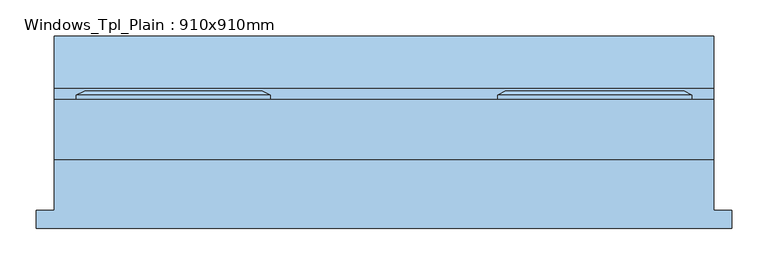
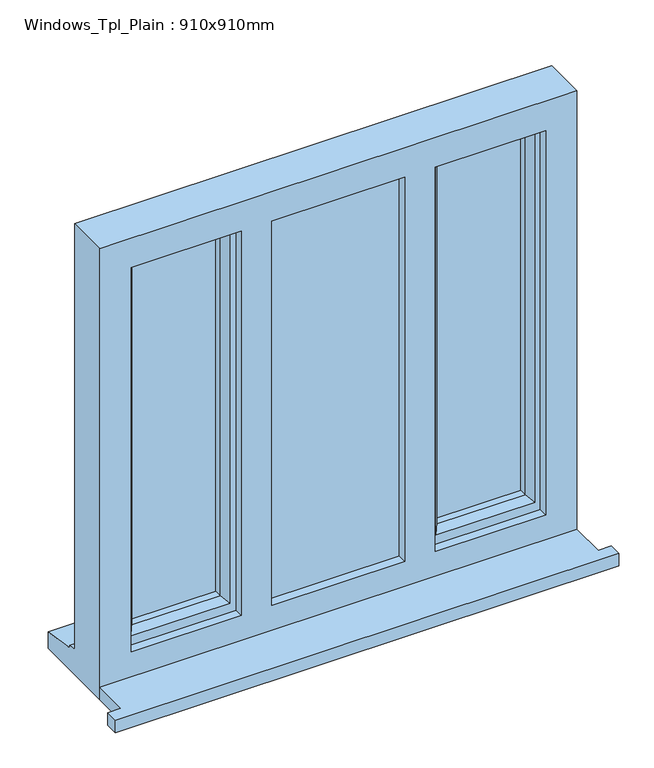
"""IFC4 building model written with IfcOpenShell, lengths in millimetres: window geometry, Windows_Tpl_Plain : 910x910mm."""

from ifc_helpers import new_model, si_unit, frame, origin, place, context, project, spatial, polyline, outline, extrude, faceted_brep, source, transform, mapped, element, save


def windows_tpl_plain_910x910mm_84e79c20(model_context):
    return source(origin(), model_context, "Body", "SolidModel", [
        extrude(outline(polyline([(-906.6666667, -118.1434322), (-906.6666667, -93.1434322), (-881.6666667, -93.1434322), (-881.6666667, -22.9434322), (28.3333333, -22.9434322), (28.3333333, -93.1434322), (53.3333333, -93.1434322), (53.3333333, -118.1434322), (-906.6666667, -118.1434322)])), frame((0.0, 0.0, 1200.0), z_axis=(0.0, 0.0, 1.0), x_axis=(1.0, 0.0, 0.0)), (0.0, 0.0, 1.0), 25.0),
        faceted_brep([(-270.0, 60.0565678, 2080.0), (-270.0, 65.8300705, 2080.0), (-270.0, 65.8300705, 1253.0), (-270.0, 60.0565678, 1253.0), (-260.0, -4.9434322, 2070.0), (-260.0, 60.0565678, 2070.0), (-260.0, 60.0565678, 1263.0), (-260.0, -4.9434322, 1263.0), (-220.0, 9.5494677, 2030.0), (-230.1480377, -4.9434322, 2040.1480377), (-230.1480377, -4.9434322, 1292.8519623), (-220.0, 9.5494677, 1303.0), (-220.0, 24.0565678, 2030.0), (-220.0, 24.0565678, 1303.0), (-230.0, 48.0565678, 2040.0), (-230.0, 24.0565678, 2040.0), (-230.0, 24.0565678, 1293.0), (-230.0, 48.0565678, 1293.0), (-220.0, 65.8300705, 2030.0), (-220.0, 48.0565678, 2030.0), (-220.0, 48.0565678, 1303.0), (-220.0, 65.8300705, 1303.0), (-237.4457548, 71.6035732, 2047.4457548), (-237.4457548, 71.6035732, 1285.5542452), (-259.2153903, 71.6035732, 2069.2153903), (-259.2153903, 71.6035732, 1263.7846097), (-1.6666667, 65.8300705, 1253.0), (-1.6666667, 60.0565678, 1253.0), (-11.6666667, 60.0565678, 1263.0), (-11.6666667, -4.9434322, 1263.0), (-41.5186289, -4.9434322, 1292.8519623), (-51.6666667, 9.5494677, 1303.0), (-51.6666667, 24.0565678, 1303.0), (-41.6666667, 24.0565678, 1293.0), (-41.6666667, 48.0565678, 1293.0), (-51.6666667, 48.0565678, 1303.0), (-51.6666667, 65.8300705, 1303.0), (-34.2209119, 71.6035732, 1285.5542452), (-12.4512764, 71.6035732, 1263.7846097), (-1.6666667, 65.8300705, 2080.0), (-1.6666667, 60.0565678, 2080.0), (-11.6666667, 60.0565678, 2070.0), (-11.6666667, -4.9434322, 2070.0), (-41.5186289, -4.9434322, 2040.1480377), (-51.6666667, 9.5494677, 2030.0), (-51.6666667, 24.0565678, 2030.0), (-41.6666667, 24.0565678, 2040.0), (-41.6666667, 48.0565678, 2040.0), (-51.6666667, 48.0565678, 2030.0), (-51.6666667, 65.8300705, 2030.0), (-34.2209119, 71.6035732, 2047.4457548), (-12.4512764, 71.6035732, 2069.2153903)], [[[0, 1, 2, 3]], [[4, 5, 6, 7]], [[8, 9, 10, 11]], [[12, 8, 11, 13]], [[14, 15, 16, 17]], [[18, 19, 20, 21]], [[22, 18, 21, 23]], [[1, 24, 25, 2]], [[3, 2, 26, 27]], [[7, 6, 28, 29]], [[11, 10, 30, 31]], [[13, 11, 31, 32]], [[17, 16, 33, 34]], [[21, 20, 35, 36]], [[23, 21, 36, 37]], [[2, 25, 38, 26]], [[27, 26, 39, 40]], [[29, 28, 41, 42]], [[31, 30, 43, 44]], [[32, 31, 44, 45]], [[34, 33, 46, 47]], [[36, 35, 48, 49]], [[37, 36, 49, 50]], [[26, 38, 51, 39]], [[40, 39, 1, 0]], [[3, 27, 40, 0], [5, 41, 28, 6]], [[42, 41, 5, 4]], [[7, 29, 42, 4], [9, 43, 30, 10]], [[44, 43, 9, 8]], [[45, 44, 8, 12]], [[15, 46, 33, 16], [13, 32, 45, 12]], [[47, 46, 15, 14]], [[17, 34, 47, 14], [19, 48, 35, 20]], [[49, 48, 19, 18]], [[50, 49, 18, 22]], [[24, 51, 38, 25], [23, 37, 50, 22]], [[39, 51, 24, 1]]]),
        faceted_brep([(-583.3333333, 60.0565678, 2080.0), (-583.3333333, 65.8300705, 2080.0), (-851.6666667, 65.8300705, 2080.0), (-851.6666667, 60.0565678, 2080.0), (-593.3333333, -4.9434322, 2070.0), (-593.3333333, 60.0565678, 2070.0), (-841.6666667, 60.0565678, 2070.0), (-841.6666667, -4.9434322, 2070.0), (-633.3333333, 9.5494677, 2030.0), (-623.1852956, -4.9434322, 2040.1480377), (-811.8147044, -4.9434322, 2040.1480377), (-801.6666667, 9.5494677, 2030.0), (-633.3333333, 24.0565678, 2030.0), (-801.6666667, 24.0565678, 2030.0), (-623.3333333, 48.0565678, 2040.0), (-623.3333333, 24.0565678, 2040.0), (-811.6666667, 24.0565678, 2040.0), (-811.6666667, 48.0565678, 2040.0), (-633.3333333, 65.8300705, 2030.0), (-633.3333333, 48.0565678, 2030.0), (-801.6666667, 48.0565678, 2030.0), (-801.6666667, 65.8300705, 2030.0), (-614.5187677, 71.6035732, 2048.8145656), (-820.4812323, 71.6035732, 2048.8145656), (-594.964114, 71.6035732, 2068.3692194), (-840.035886, 71.6035732, 2068.3692194), (-851.6666667, 65.8300705, 1253.0), (-851.6666667, 60.0565678, 1253.0), (-841.6666667, 60.0565678, 1263.0), (-841.6666667, -4.9434322, 1263.0), (-811.8147044, -4.9434322, 1292.8519623), (-801.6666667, 9.5494677, 1303.0), (-801.6666667, 24.0565678, 1303.0), (-811.6666667, 24.0565678, 1293.0), (-811.6666667, 48.0565678, 1293.0), (-801.6666667, 48.0565678, 1303.0), (-801.6666667, 65.8300705, 1303.0), (-820.4812323, 71.6035732, 1284.1854344), (-840.035886, 71.6035732, 1264.6307806), (-583.3333333, 65.8300705, 1253.0), (-583.3333333, 60.0565678, 1253.0), (-593.3333333, 60.0565678, 1263.0), (-593.3333333, -4.9434322, 1263.0), (-623.1852956, -4.9434322, 1292.8519623), (-633.3333333, 9.5494677, 1303.0), (-633.3333333, 24.0565678, 1303.0), (-623.3333333, 24.0565678, 1293.0), (-623.3333333, 48.0565678, 1293.0), (-633.3333333, 48.0565678, 1303.0), (-633.3333333, 65.8300705, 1303.0), (-614.5187677, 71.6035732, 1284.1854344), (-594.964114, 71.6035732, 1264.6307806)], [[[0, 1, 2, 3]], [[4, 5, 6, 7]], [[8, 9, 10, 11]], [[12, 8, 11, 13]], [[14, 15, 16, 17]], [[18, 19, 20, 21]], [[22, 18, 21, 23]], [[1, 24, 25, 2]], [[3, 2, 26, 27]], [[7, 6, 28, 29]], [[11, 10, 30, 31]], [[13, 11, 31, 32]], [[17, 16, 33, 34]], [[21, 20, 35, 36]], [[23, 21, 36, 37]], [[2, 25, 38, 26]], [[27, 26, 39, 40]], [[0, 3, 27, 40], [41, 28, 6, 5]], [[29, 28, 41, 42]], [[4, 7, 29, 42], [43, 30, 10, 9]], [[31, 30, 43, 44]], [[32, 31, 44, 45]], [[46, 33, 16, 15], [12, 13, 32, 45]], [[34, 33, 46, 47]], [[14, 17, 34, 47], [48, 35, 20, 19]], [[36, 35, 48, 49]], [[37, 36, 49, 50]], [[51, 38, 25, 24], [22, 23, 37, 50]], [[26, 38, 51, 39]], [[40, 39, 1, 0]], [[42, 41, 5, 4]], [[44, 43, 9, 8]], [[45, 44, 8, 12]], [[47, 46, 15, 14]], [[49, 48, 19, 18]], [[50, 49, 18, 22]], [[39, 51, 24, 1]]]),
        faceted_brep([(28.3333333, -22.9434322, 2110.0), (-881.6666667, -22.9434322, 2110.0), (-881.6666667, -22.9434322, 1200.0), (28.3333333, -22.9434322, 1200.0), (-31.6666667, -22.9434322, 2050.0), (-31.6666667, -22.9434322, 1275.0), (-242.0, -22.9434322, 1275.0), (-242.0, -22.9434322, 2050.0), (-300.0, -22.9434322, 2050.0), (-300.0, -22.9434322, 1275.0), (-553.3333333, -22.9434322, 1275.0), (-553.3333333, -22.9434322, 2050.0), (-611.3333333, -22.9434322, 2050.0), (-611.3333333, -22.9434322, 1275.0), (-821.6666667, -22.9434322, 1275.0), (-821.6666667, -22.9434322, 2050.0), (-881.6666667, 60.0565678, 2110.0), (-881.6666667, 60.0565678, 1251.0), (-881.6666667, 75.0565678, 1249.68767), (-881.6666667, 75.0565678, 1244.7449676), (-881.6666667, 147.5565678, 1233.8088847), (-881.6666667, 147.5565678, 1200.0), (28.3333333, 60.0565678, 2110.0), (28.3333333, 60.0565678, 1251.0), (-841.6666667, 60.0565678, 2070.0), (-841.6666667, 60.0565678, 1263.0), (-593.3333333, 60.0565678, 1263.0), (-593.3333333, 60.0565678, 2070.0), (-553.3333333, 60.0565678, 2070.0), (-553.3333333, 60.0565678, 1263.0), (-300.0, 60.0565678, 1263.0), (-300.0, 60.0565678, 2070.0), (-260.0, 60.0565678, 2070.0), (-260.0, 60.0565678, 1263.0), (-11.6666667, 60.0565678, 1263.0), (-11.6666667, 60.0565678, 2070.0), (-841.6666667, -4.9434322, 2070.0), (-841.6666667, -4.9434322, 1263.0), (-563.3333333, -4.9434322, 2070.0), (-290.0, -4.9434322, 2070.0), (-290.0, -4.9434322, 1263.0), (-563.3333333, -4.9434322, 1263.0), (-300.0, -4.9434322, 2050.0), (-553.3333333, -4.9434322, 2050.0), (-553.3333333, -4.9434322, 1275.0), (-300.0, -4.9434322, 1275.0), (-260.0, -4.9434322, 2070.0), (-11.6666667, -4.9434322, 2070.0), (-11.6666667, -4.9434322, 1263.0), (-260.0, -4.9434322, 1263.0), (-31.6666667, -4.9434322, 2050.0), (-242.0, -4.9434322, 2050.0), (-242.0, -4.9434322, 1275.0), (-31.6666667, -4.9434322, 1275.0), (-593.3333333, -4.9434322, 2070.0), (-593.3333333, -4.9434322, 1263.0), (-611.3333333, -4.9434322, 2050.0), (-821.6666667, -4.9434322, 2050.0), (-821.6666667, -4.9434322, 1275.0), (-611.3333333, -4.9434322, 1275.0), (-553.3333333, 19.0565678, 2070.0), (-300.0, 19.0565678, 2070.0), (-290.0, 19.0565678, 2070.0), (-563.3333333, 19.0565678, 2070.0), (28.3333333, 147.5565678, 1200.0), (28.3333333, 147.5565678, 1233.8088847), (28.3333333, 75.0565678, 1244.7449676), (28.3333333, 75.0565678, 1249.68767), (-553.3333333, 19.0565678, 1263.0), (-563.3333333, 19.0565678, 1263.0), (-290.0, 19.0565678, 1263.0), (-300.0, 19.0565678, 1263.0)], [[[0, 1, 2, 3], [4, 5, 6, 7], [8, 9, 10, 11], [12, 13, 14, 15]], [[2, 1, 16, 17, 18, 19, 20, 21]], [[17, 16, 22, 23], [24, 25, 26, 27], [28, 29, 30, 31], [32, 33, 34, 35]], [[25, 24, 36, 37]], [[38, 39, 40, 41], [42, 43, 44, 45]], [[46, 47, 48, 49], [50, 51, 52, 53]], [[36, 54, 55, 37], [56, 57, 58, 59]], [[57, 15, 14, 58]], [[1, 0, 22, 16]], [[36, 24, 27, 54]], [[35, 47, 46, 32]], [[60, 28, 31, 61, 62, 39, 38, 63]], [[15, 57, 56, 12]], [[50, 4, 7, 51]], [[11, 43, 42, 8]], [[23, 22, 0, 3, 64, 65, 66, 67]], [[35, 34, 48, 47]], [[4, 50, 53, 5]], [[43, 11, 10, 44]], [[12, 56, 59, 13]], [[27, 26, 55, 54]], [[29, 28, 60, 68]], [[68, 60, 63, 69]], [[69, 63, 38, 41]], [[62, 70, 40, 39]], [[70, 62, 61, 71]], [[71, 61, 31, 30]], [[33, 32, 46, 49]], [[51, 7, 6, 52]], [[8, 42, 45, 9]], [[64, 3, 2, 21]], [[65, 64, 21, 20]], [[66, 65, 20, 19]], [[67, 66, 19, 18]], [[23, 67, 18, 17]], [[26, 25, 37, 55]], [[34, 33, 49, 48]], [[41, 40, 70, 71, 30, 29, 68, 69]], [[6, 5, 53, 52]], [[45, 44, 10, 9]], [[59, 58, 14, 13]]]),
        extrude(outline(polyline([(-623.3333333, 24.0565678), (-811.6666667, 24.0565678), (-811.6666667, 48.0565678), (-623.3333333, 48.0565678), (-623.3333333, 24.0565678)])), frame((0.0, 0.0, 1293.0), z_axis=(0.0, 0.0, 1.0), x_axis=(1.0, 0.0, 0.0)), (0.0, 0.0, 1.0), 747.0),
        extrude(outline(polyline([(-563.3333333, 19.0565678), (-290.0, 19.0565678), (-290.0, -4.9434322), (-563.3333333, -4.9434322), (-563.3333333, 19.0565678)])), frame((0.0, 0.0, 1263.0), z_axis=(0.0, 0.0, 1.0), x_axis=(1.0, 0.0, 0.0)), (0.0, 0.0, 1.0), 807.0),
        extrude(outline(polyline([(-41.6666667, 24.0565678), (-230.0, 24.0565678), (-230.0, 48.0565678), (-41.6666667, 48.0565678), (-41.6666667, 24.0565678)])), frame((0.0, 0.0, 1293.0), z_axis=(0.0, 0.0, 1.0), x_axis=(1.0, 0.0, 0.0)), (0.0, 0.0, 1.0), 747.0),
    ])


if __name__ == "__main__":
    model = new_model("IFC4")
    model_context = context("Model", 3, world=origin())
    ifc_project = project(units=[si_unit("LENGTHUNIT", "METRE", prefix="MILLI")], contexts=[model_context])
    site = spatial("IfcSite", under=ifc_project)
    building = spatial("IfcBuilding", under=site)
    placement = place(None, origin())
    windows_tpl_plain_910x910mm_shape = windows_tpl_plain_910x910mm_84e79c20(model_context)
    element("IfcWindow", 1, ObjectType="Windows_Tpl_Plain : 910x910mm", at=placement, inside=building, context=model_context, shape_type="MappedRepresentation", body=[
        mapped(windows_tpl_plain_910x910mm_shape, transform((0.0, 0.0, 0.0), x_axis=(1.0, 0.0, 0.0), y_axis=(0.0, 1.0, 0.0), z_axis=(0.0, 0.0, 1.0))),
    ])
    save(model, "model.ifc")

# Revit data of these elements
# Type "Windows_Tpl_Plain : 910x910mm"
#   Type Mark = "18"
#   Operation = "TriplePanelVertical"
#   Construction Type Id = "GSP4R"
#   Manufacturer = "Revit"
#   Keynote = "L10"
#   Analytic Construction = "1/8 in Pilkington single glazing"
#   Wrap Layers (Ext) from Ext = 0' - 4.03543"
#   Wrap Layers (Int) from Ext = 0' - 6.98819"
#   Window Board Projection = 0' - 0.98425"
#   Window Board Extension = 0' - 0.98425"
#   Visual Light Transmittance = 0.9
#   Solar Heat Gain Coefficient = 0.78
#   Rough Width = 2' - 11.82677"
#   Rough Height = 2' - 11.82677"
#   Height = 2' - 11.82677"
#   Width = 2' - 11.82677"
#   Heat Transfer Coefficient (U) = 0.6496 BTU/(h·ft²·°F)
#   Glazing Thickness = 0' - 0.94488"
#   FrameOffset - External = 0' - 1.9685"
#   Frame Depth = 0' - 2.55906"
#   Default Head Height = 6' - 11.07087"
#   Cill Depth = 0' - 3.44488"
#   Cavity Closer Width = 0' - 1.9685"
#   Cavity Closer Offset from Ext = 0' - 4.03543"
#   Cavity Closer Depth = 0' - 3.34646"
#   Vis - Cavity Closers = yes
#   Define Thermal Properties by = 1
#   Material Trim = Window Frame
#   Material Glass = Glass
#   Material Frame = Window Frame
#   Wall Closure = (empty or 0)
# Element 1 (IfcWindow, "Windows_Tpl_Plain : 910x910mm")
#   Materials on its faces: "Window Frame", "Glass"
# Materials
#   "Window Frame": colour RGB 249 249 249, transparency 0
#   "Glass": class "Glass", colour RGB 0 128 192, transparency 0.75, Description = "Soda Lime Glass", Cost = 0
